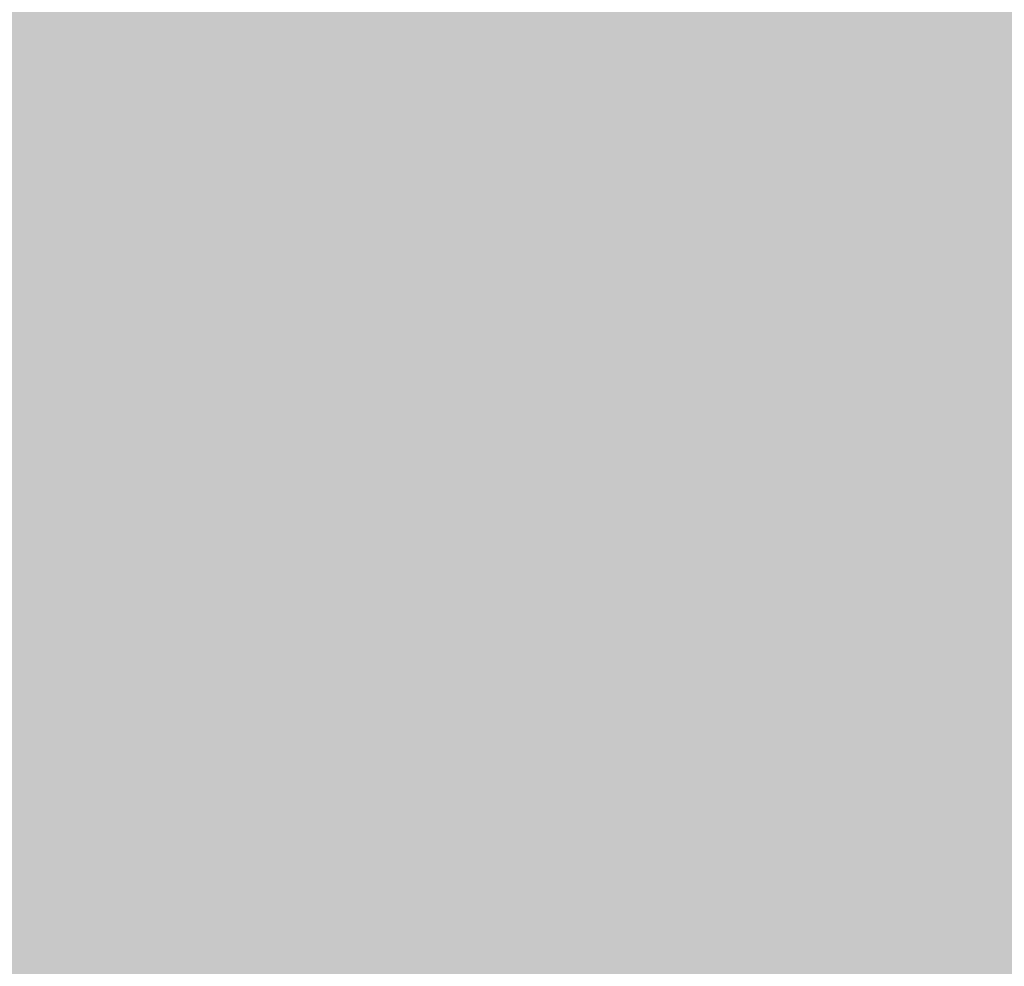
# Model space of a CAD drawing. Units: inches. Extents: x 2083 to 3317, y 1141 to 2115.
# Tile 140 of 256: x 3126.1318 to 3126.6699, y 1263.6134 to 1264.1307. Entities that reach past the tile are written whole.
import ezdxf

# ---------------------------------------------------------------- set-up
doc = ezdxf.new("R2010")
doc.units = ezdxf.units.IN
doc.layers.add('A-ANNO-DIMS', color=2, linetype='Continuous', lineweight=18)
doc.layers.add('A-WALL-PATT', color=251, linetype='Continuous', lineweight=13, true_color=0x636466)
doc.styles.get("Standard").update_dxf_attribs({"font": 'arial.ttf'})
doc.dimstyles.new('ISO-25', dxfattribs={"dimtxt": 12, "dimasz": 12, "dimexe": 1.25, "dimexo": 0.625, "dimtad": 1, "dimlunit": 3, "dimtxsty": 'Standard', "dimcen": 2.5, "dimadec": 0, "dimazin": 0, "dimtfac": 1, "dimtmove": 0, "dimatfit": 3, "dimfxl": 1, "dimarcsym": 0})

# ---------------------------------------------------------------- blocks, each defined once
blk = doc.blocks.new('*D26')
at = {"layer": 'A-ANNO-DIMS', "color": 0, "lineweight": -2, "transparency": 16777216}
for p, q in [((3088.98584, 1274.91509), (3088.98584, 1270.95196)), ((3111.24004, 1274.91509), (3111.24004, 1270.95196)), ((3076.98584, 1272.20196), (2840.26245, 1272.20196)), ((3111.24004, 1272.20196), (3088.98584, 1272.20196)), ((3123.24004, 1272.20196), (3135.24004, 1272.20196))]:
    blk.add_line(p, q, dxfattribs=at)
at = {"layer": 'A-ANNO-DIMS', "color": 0, "transparency": 16777216}
for points in [[(3076.98584, 1274.20196), (3076.98584, 1270.20196), (3088.98584, 1272.20196)], [(3123.24004, 1274.20196), (3123.24004, 1270.20196), (3111.24004, 1272.20196)]]:
    blk.add_solid(points, dxfattribs=at)
at = {"layer": 'Defpoints', "color": 0, "transparency": 16777216}
for p in [(3088.98584, 1275.54009), (3111.24004, 1275.54009), (3088.98584, 1272.20196)]:
    blk.add_point(p, dxfattribs=at)
at = {"layer": 'A-ANNO-DIMS', "color": 0, "transparency": 16777216, "insert": (2952.62415, 1279.0316), "char_height": 12, "attachment_point": 5}
blk.add_mtext('NIGHTSTAND 1\'-10 1/2" TYP.', dxfattribs=at)
blk = doc.blocks.new('*D27')
at = {"layer": 'A-ANNO-DIMS', "color": 0, "lineweight": -2, "transparency": 16777216}
for p, q in [((3114.57817, 1309.79428), (3114.57817, 1321.79428)), ((3111.86504, 1297.79428), (3115.82817, 1297.79428)), ((3114.57817, 1297.79428), (3114.57817, 1275.54009)), ((3111.86504, 1275.54009), (3115.82817, 1275.54009)), ((3114.57817, 1263.54009), (3114.57817, 1140.98859))]:
    blk.add_line(p, q, dxfattribs=at)
at = {"layer": 'A-ANNO-DIMS', "color": 0, "transparency": 16777216}
for points in [[(3112.57817, 1309.79428), (3116.57817, 1309.79428), (3114.57817, 1297.79428)], [(3112.57817, 1263.54009), (3116.57817, 1263.54009), (3114.57817, 1275.54009)]]:
    blk.add_solid(points, dxfattribs=at)
at = {"layer": 'Defpoints', "color": 0, "transparency": 16777216}
for p in [(3111.24004, 1297.79428), (3111.24004, 1275.54009), (3114.57817, 1275.54009)]:
    blk.add_point(p, dxfattribs=at)
at = {"layer": 'A-ANNO-DIMS', "color": 0, "transparency": 16777216, "insert": (3107.74853, 1196.26434), "char_height": 12, "attachment_point": 5, "rotation": 90}
blk.add_mtext('1\'-10 1/2" TYP.', dxfattribs=at)

msp = doc.modelspace()

# ---------------------------------------------------------------- hatches: boundary and pattern name
at = {"layer": 'A-WALL-PATT'}
h = msp.add_hatch(color=256, dxfattribs=at)
h.dxf.hatch_style = 1
h.paths.add_polyline_path([(3126.95978, 2020.76136), (2748.95978, 2020.76136), (2604.95978, 2020.76136), (2226.95978, 2020.76136), (2226.95978, 1702.76136), (2466.95978, 1702.76136), (2466.95978, 1582.76136), (2418.95978, 1582.76136), (2418.95978, 1477.76136), (2226.95978, 1477.76136), (2226.95978, 1263.26136), (2544.95978, 1263.26136), (2544.95978, 1411.76136), (2604.95978, 1411.76136), (2685.95978, 1411.76136), (2685.95978, 1420.76136), (2604.95978, 1420.76136), (2604.95978, 1573.76136), (2604.95978, 1702.76136), (2604.95978, 2011.76136), (2748.95978, 2011.76136), (2748.95978, 1702.76136), (2862.95978, 1702.76136), (2862.95978, 1621.76136), (2871.95978, 1621.76136), (2871.95978, 1702.76136), (2883.95978, 1702.76136), (2883.95978, 1706.93946, -0.026459), (2883.95978, 1711.76136), (2757.95978, 1711.76136), (2757.95978, 1807.76136), (2787.95978, 1807.76136), (2787.95978, 1812.26136), (2757.95978, 1812.26136), (2757.95978, 2011.76136), (2877.95978, 2011.76136), (2877.95978, 1812.26136), (2847.95978, 1812.26136), (2847.95978, 1807.76136), (2889.83574, 1807.76136), (2889.83574, 1812.26136), (2882.45978, 1812.26136), (2882.45978, 2011.76136), (3117.95978, 2011.76136), (3117.95978, 1812.26136), (2937.83574, 1812.26136), (2937.83574, 1807.76136), (2995.70978, 1807.76136), (2995.70978, 1796.11767), (3000.20978, 1796.11767), (3000.20978, 1807.76136), (3117.95978, 1807.76136), (3117.95978, 1711.76136), (3000.20978, 1711.76136), (3000.20978, 1760.11767), (2998.5727, 1760.11767, -0.020711), (2995.70978, 1760.11767), (2995.70978, 1711.76136), (2931.95978, 1711.76136), (2931.95978, 1702.76136), (3126.95978, 1702.76136)])
h.paths.add_polyline_path([(2471.45978, 2011.76136), (2471.45978, 1810.01136), (2462.71694, 1810.01136), (2462.71694, 1805.51136), (2505.95978, 1805.51136), (2505.95978, 1810.01136), (2475.95978, 1810.01136), (2475.95978, 2011.76136), (2595.95978, 2011.76136), (2595.95978, 1810.01136), (2565.95978, 1810.01136), (2565.95978, 1805.51136), (2595.95978, 1805.51136), (2595.95978, 1711.76136), (2235.95978, 1711.76136), (2235.95978, 1805.51136), (2353.70978, 1805.51136), (2353.70978, 1796.05416), (2358.20978, 1796.05416), (2358.20978, 1805.51136), (2414.71694, 1805.51136), (2414.71694, 1810.01136), (2235.95978, 1810.01136), (2235.95978, 2011.76136)], flags=16)
h.paths.add_polyline_path([(2270.20473, 1994.61001), (2270.20473, 1970.61001), (2246.20473, 1970.61001), (2246.20473, 1994.61001)], flags=0)
edge = h.paths.add_edge_path(flags=0)
edge.add_ellipse((2332.02739, 1899.79818), major_axis=(-3.04299, 3.04299), ratio=0.1682525, start_angle=-161.33217, end_angle=-156.30711, ccw=False)
edge.add_ellipse((2333.08204, 1898.74353), major_axis=(-1.05465, 1.05465), ratio=0.4535321, start_angle=-123.37102, end_angle=-94.15911)
edge = h.paths.add_edge_path(flags=0)
edge.add_ellipse((2332.02739, 1968.87629), major_axis=(3.04299, 3.04299), ratio=0.1682525, start_angle=18.66783, end_angle=23.69289)
edge.add_spline(control_points=[(2332.9256, 1970.6911), (2332.22677, 1970.3361), (2330.89371, 1969.65891), (2328.41308, 1970.93214), (2327.20393, 1967.74871), (2324.7096, 1969.95559), (2322.53282, 1967.01235), (2320.01285, 1971.29581), (2317.68031, 1968.15784), (2316.04053, 1967.10205), (2315.4269, 1966.8096)], knot_values=[0, 0, 0, 0, 2.267059, 4.324559, 6.685584, 8.878641, 11.121502, 14.300359, 17.755284, 19.732645, 19.732645, 19.732645, 19.732645], degree=3, periodic=0)
edge.add_ellipse((2332.02739, 1968.87629), major_axis=(3.04299, 3.04299), ratio=0.1682525, start_angle=18.66783, end_angle=23.69289, ccw=False)
edge.add_ellipse((2333.08204, 1969.93094), major_axis=(1.05465, 1.05465), ratio=0.4535321, start_angle=56.62898, end_angle=85.84089, ccw=False)
edge = h.paths.add_edge_path(flags=0)
edge.add_spline(control_points=[(2296.42829, 1967.98791), (2293.6278, 1965.33631), (2287.70362, 1959.72709), (2299.74386, 1949.9957), (2294.53259, 1935.66853), (2290.57323, 1920.60351), (2293.39412, 1909.97369), (2296.18541, 1904.96654)], knot_values=[0.099185, 0.099185, 0.099185, 0.099185, 0.345301, 0.619822, 0.982653, 1.386093, 1.810555, 1.810555, 1.810555, 1.810555], degree=3, periodic=0)
edge.add_spline(control_points=[(2296.18541, 1904.96654), (2297.38358, 1902.6193), (2298.00097, 1901.94931), (2298.55297, 1901.46815)], knot_values=[0.006246, 0.006246, 0.006246, 0.006246, 0.055476, 0.055476, 0.055476, 0.055476], degree=3, periodic=0)
edge.add_spline(control_points=[(2298.55297, 1901.46815), (2297.25861, 1900.92322), (2295.22529, 1900.23213), (2293.06023, 1900.61421), (2292.10142, 1900.78841), (2292.08958, 1900.79057)], knot_values=[0.312835, 0.312835, 0.312835, 0.312835, 0.40178, 0.474987, 0.475903, 0.475903, 0.475903, 0.475903], degree=3, periodic=0)
edge.add_arc((2292.79365, 1904.66411), 3.93701, 215.4209, 259.69818, ccw=False)
edge.add_spline(control_points=[(2289.58531, 1902.3823), (2289.47665, 1902.53509), (2289.36848, 1902.68804), (2289.26086, 1902.84117)], knot_values=[0.102872, 0.102872, 0.102872, 0.102872, 0.116896, 0.116896, 0.116896, 0.116896], degree=3, periodic=0)
edge.add_spline(control_points=[(2289.26086, 1902.84117), (2288.6866, 1902.55019), (2287.64005, 1902.0199), (2285.88134, 1901.87395), (2283.85297, 1901.50435), (2281.71999, 1899.71054), (2278.46699, 1899.49294), (2276.15714, 1901.8832), (2272.25895, 1899.80407), (2267.77761, 1901.84318), (2262.24388, 1900.18403), (2257.41493, 1901.78206), (2254.31837, 1900.72612), (2253.17828, 1900.33734)], knot_values=[0, 0, 0, 0, 1.907977, 3.477176, 5.261074, 7.972851, 11.680248, 13.717921, 16.939592, 22.789562, 27.502503, 33.595215, 37.145618, 37.145618, 37.145618, 37.145618], degree=3, periodic=0)
edge.add_line((2253.17828, 1900.33734), (2250.24424, 1902.84117))
edge.add_line((2250.24424, 1902.84117), (2250.24424, 1965.8333))
edge.add_line((2250.24424, 1965.8333), (2253.17828, 1968.33712))
edge.add_spline(control_points=[(2253.17828, 1968.33712), (2254.31837, 1967.94835), (2257.41493, 1966.89241), (2262.24388, 1968.49043), (2267.77761, 1966.83128), (2271.52673, 1968.53722), (2273.87591, 1967.82829), (2274.2067, 1967.72764)], knot_values=[0, 0, 0, 0, 0.09018, 0.244935, 0.364644, 0.513233, 0.537855, 0.537855, 0.537855, 0.537855], degree=3, periodic=0)
edge.add_arc((2274.35289, 1963.79335), 3.93701, 72.05113, 92.12795, ccw=False)
edge.add_arc((2281.29693, 1985.23), 18.5963, 252.051134, 288.565722)
edge.add_arc((2292.31672, 1956.02888), 12.64608, 71.026788, 113.778218, ccw=False)
edge = h.paths.add_edge_path(flags=0)
edge.add_spline(control_points=[(2274.89941, 1951.85619), (2275.06616, 1951.61659), (2275.23269, 1951.37659), (2275.39799, 1951.13585)], knot_values=[1.409916, 1.409916, 1.409916, 1.409916, 1.43159, 1.43159, 1.43159, 1.43159], degree=3, periodic=0)
edge.add_spline(control_points=[(2275.39799, 1951.13585), (2275.79211, 1950.56189), (2276.17923, 1949.98377), (2276.54555, 1949.3971)], knot_values=[1.358238, 1.358238, 1.358238, 1.358238, 1.409916, 1.409916, 1.409916, 1.409916], degree=3, periodic=0)
edge.add_line((2276.54555, 1949.3971), (2277.43729, 1947.86218))
edge.add_spline(control_points=[(2277.43729, 1947.86218), (2276.30383, 1945.67311), (2274.6397, 1942.42688), (2274.63161, 1938.0939), (2272.79912, 1930.85155), (2274.35643, 1943.89705), (2275.94768, 1947.92336), (2276.54555, 1949.3971)], knot_values=[0.005632, 0.005632, 0.005632, 0.005632, 0.186014, 0.266002, 0.357087, 0.59639, 0.739732, 0.739732, 0.739732, 0.739732], degree=3, periodic=0)
edge.add_spline(control_points=[(2276.54555, 1949.3971), (2276.17923, 1949.98377), (2275.79211, 1950.56189), (2275.39799, 1951.13585)], knot_values=[1.358238, 1.358238, 1.358238, 1.358238, 1.409916, 1.409916, 1.409916, 1.409916], degree=3, periodic=0)
edge.add_spline(control_points=[(2275.39799, 1951.13585), (2274.9425, 1950.08045), (2274.20776, 1948.02527), (2273.9346, 1944.85148), (2272.46853, 1937.62749), (2273.46622, 1945.69647), (2274.70062, 1951.05947), (2274.89941, 1951.85619)], knot_values=[0.104364, 0.104364, 0.104364, 0.104364, 0.189636, 0.269624, 0.36071, 0.600013, 0.644622, 0.644622, 0.644622, 0.644622], degree=3, periodic=0)
h.paths.add_polyline_path([(2269.16751, 1963.12757, -0.357527), (2268.17063, 1960.97637, -0.092561), (2268.17063, 1939.43632, -0.357527), (2269.16751, 1937.28512, -0.357527), (2267.01631, 1938.282, -0.164785), (2254.68558, 1938.282, -0.357527), (2252.53438, 1937.28512, -0.357527), (2253.53126, 1939.43632, -0.092561), (2253.53126, 1960.97637, -0.357527), (2252.53438, 1963.12757, -0.357527), (2254.68558, 1962.13069, -0.164785), (2267.01631, 1962.13069, -0.357527)], flags=0)
h.paths.add_polyline_path([(2248.87407, 1967.8018), (2248.87407, 1957.02771), (2249.45778, 1957.02771), (2249.45778, 1911.64676), (2248.87407, 1911.64676), (2248.87407, 1900.87267), (2246.51186, 1900.87267, 0.197327), (2244.14966, 1902.45687), (2244.14966, 1966.21759, 0.197327), (2246.51186, 1967.8018)], flags=0)
h.paths.add_polyline_path([(2269.16751, 1931.38934, -0.357527), (2268.17063, 1929.23814, -0.092561), (2268.17063, 1907.6981, -0.357527), (2269.16751, 1905.54689, -0.357527), (2267.01631, 1906.54377, -0.164785), (2254.68558, 1906.54377, -0.357527), (2252.53438, 1905.54689, -0.357527), (2253.53126, 1907.6981, -0.092561), (2253.53126, 1929.23814, -0.357527), (2252.53438, 1931.38934, -0.357527), (2254.68558, 1930.39246, -0.164785), (2267.01631, 1930.39246, -0.357527)], flags=0)
edge = h.paths.add_edge_path(flags=0)
edge.add_spline(control_points=[(2276.19686, 1906.7237), (2276.16814, 1909.02893), (2276.11405, 1913.37185), (2270.59842, 1924.92498), (2273.90517, 1919.01278), (2275.92171, 1916.26206), (2275.47457, 1912.40215), (2277.25787, 1910.38062), (2276.69604, 1908.22504), (2276.64622, 1906.81302), (2276.61782, 1906.00841)], knot_values=[0, 0, 0, 0, 8.61026, 16.221274, 18.843057, 23.804898, 27.440828, 29.356102, 31.203478, 33.650687, 33.650687, 33.650687, 33.650687], degree=3, periodic=0)
edge.add_spline(control_points=[(2276.61782, 1906.00841), (2276.62331, 1905.62414), (2276.49774, 1904.62866), (2275.44178, 1903.85473), (2274.93731, 1903.08045), (2274.85908, 1902.84117)], knot_values=[0.156488, 0.156488, 0.156488, 0.156488, 0.184398, 0.231376, 0.250598, 0.250598, 0.250598, 0.250598], degree=3, periodic=0)
edge.add_line((2274.85908, 1902.84117), (2276.50598, 1902.84117))
edge.add_spline(control_points=[(2276.50598, 1902.84117), (2276.78831, 1903.08494), (2277.66507, 1904.1252), (2278.24954, 1904.34074), (2277.65387, 1908.52739), (2278.15567, 1906.22781), (2278.10046, 1905.28595), (2278.84667, 1904.06901), (2277.85679, 1903.41495), (2277.87419, 1902.99105), (2277.90356, 1902.84117)], knot_values=[0.059574, 0.059574, 0.059574, 0.059574, 0.080753, 0.103741, 0.16972, 0.176036, 0.207137, 0.240474, 0.262341, 0.27366, 0.27366, 0.27366, 0.27366], degree=3, periodic=0)
edge.add_line((2277.90356, 1902.84117), (2280.02983, 1902.84117))
edge.add_spline(control_points=[(2280.02983, 1902.84117), (2279.88822, 1903.0884), (2279.49926, 1903.98155), (2280.15228, 1905.93935), (2278.10362, 1909.65776), (2279.76239, 1907.18529), (2280.3279, 1904.87486), (2280.48511, 1903.48959), (2281.46327, 1903.24943), (2281.75834, 1902.9365), (2281.83404, 1902.84117)], knot_values=[0.013856, 0.013856, 0.013856, 0.013856, 0.034874, 0.088867, 0.107879, 0.126738, 0.158714, 0.193757, 0.217487, 0.226722, 0.226722, 0.226722, 0.226722], degree=3, periodic=0)
edge.add_spline(control_points=[(2281.83404, 1902.84117), (2281.78753, 1902.8267), (2281.64702, 1902.78299), (2281.39553, 1902.85949), (2281.08808, 1902.98524), (2280.72068, 1903.0609), (2280.33345, 1903.02573), (2280.12477, 1902.89888), (2280.02983, 1902.84117)], knot_values=[0, 0, 0, 0, 0.14413, 0.435517, 0.749276, 1.153046, 1.548371, 1.878348, 1.878348, 1.878348, 1.878348], degree=3, periodic=0)
edge.add_line((2280.02983, 1902.84117), (2277.90356, 1902.84117))
edge.add_spline(control_points=[(2277.90356, 1902.84117), (2277.89286, 1902.79586), (2277.8654, 1902.67964), (2277.60748, 1902.68748), (2277.27405, 1902.8007), (2276.83792, 1902.61977), (2276.58381, 1902.78926), (2276.50598, 1902.84117)], knot_values=[0, 0, 0, 0, 0.127189, 0.326199, 0.628009, 1.24357, 1.515331, 1.515331, 1.515331, 1.515331], degree=3, periodic=0)
edge.add_line((2276.50598, 1902.84117), (2274.85908, 1902.84117))
edge.add_spline(control_points=[(2274.85908, 1902.84117), (2274.81444, 1902.89859), (2274.72513, 1903.01345), (2274.49348, 1903.11897), (2274.24429, 1902.96054), (2273.93712, 1903.18494), (2273.61404, 1902.98314), (2273.40832, 1902.88304), (2273.32225, 1902.84117)], knot_values=[0, 0, 0, 0, 0.21843, 0.436957, 0.687977, 0.990379, 1.398396, 1.69185, 1.69185, 1.69185, 1.69185], degree=3, periodic=0)
edge.add_spline(control_points=[(2273.32225, 1902.84117), (2273.61674, 1903.44569), (2274.274, 1904.53825), (2276.02724, 1904.5737), (2276.20696, 1906.58364), (2276.19686, 1906.7237)], knot_values=[0.012227, 0.012227, 0.012227, 0.012227, 0.059472, 0.106218, 0.134458, 0.134458, 0.134458, 0.134458], degree=3, periodic=0)
h.paths.add_polyline_path([(2270.77605, 1897.78983), (2270.77605, 1873.78983), (2246.77605, 1873.78983), (2246.77605, 1897.78983)], flags=0)
h.paths.add_polyline_path([(2353.70978, 1760.00506), (2353.70978, 1760.05416), (2358.20978, 1760.05416, -0.033729)], flags=0)
h.paths.add_polyline_path([(2321.81912, 1737.52919), (2341.99533, 1737.52919, -0.414214), (2343.20327, 1736.32124), (2343.20327, 1721.0206, -0.414214), (2341.99533, 1719.81265), (2321.81912, 1719.81265, -0.414214), (2320.61117, 1721.0206), (2320.61117, 1736.32124, -0.414214)], flags=0)
h.paths.add_polyline_path([(2324.23501, 1736.32124), (2339.57944, 1736.32124, -0.414214), (2341.99533, 1733.90535), (2341.99533, 1725.44973, -0.414214), (2339.57944, 1723.03384), (2333.68059, 1723.03384), (2333.84532, 1722.04547, -0.870646), (2335.4254, 1721.82589, -0.767327), (2333.92269, 1721.42324), (2331.29102, 1721.42324, -0.767327), (2329.78832, 1721.82589, -0.870646), (2331.3684, 1722.04547), (2331.53313, 1723.03384), (2324.23501, 1723.03384, -0.414214), (2321.81912, 1725.44973), (2321.81912, 1733.90535, -0.414214)], flags=0)
h.paths.add_polyline_path([(2570.48379, 1928.61544), (2589.68379, 1928.61544), (2590.16883, 1928.61544), (2590.16883, 1904.9934), (2570.48379, 1904.9934)], flags=0)
h.paths.add_polyline_path([(2574.44732, 1927.26382, -1), (2572.82884, 1927.26382, -1)], flags=0)
h.paths.add_polyline_path([(2573.08987, 1926.94088), (2573.92503, 1927.77604), (2574.14774, 1927.55333), (2573.31258, 1926.71817)], flags=0)
h.paths.add_polyline_path([(2578.77906, 1919.72962, -1), (2571.59166, 1919.72962, -1)], flags=0)
h.paths.add_polyline_path([(2578.38536, 1919.72962, -1), (2571.98536, 1919.72962, -1)], flags=0)
h.paths.add_polyline_path([(2331.59576, 1729.47622, -1), (2333.61795, 1729.47622, -1)], flags=0)
h.paths.add_polyline_path([(2578.03423, 1927.26382, -1), (2576.41574, 1927.26382, -1)], flags=0)
h.paths.add_polyline_path([(2576.68885, 1927.53109), (2576.91156, 1927.7538), (2577.74673, 1926.91863), (2577.52402, 1926.69592)], flags=0)
h.paths.add_polyline_path([(2578.13906, 1909.85954, -1), (2572.23166, 1909.85954, -1)], flags=0)
h.paths.add_polyline_path([(2577.74536, 1909.85954, -1), (2572.62536, 1909.85954, -1)], flags=0)
h.paths.add_polyline_path([(2583.79772, 1927.26382, -1), (2582.17923, 1927.26382, -1)], flags=0)
h.paths.add_polyline_path([(2582.71865, 1927.7538), (2583.55381, 1926.91863), (2583.3311, 1926.69592), (2582.49594, 1927.53109)], flags=0)
h.paths.add_polyline_path([(2582.49594, 1927.53109), (2582.71865, 1927.7538), (2583.55381, 1926.91863), (2583.3311, 1926.69592)], flags=0)
h.paths.add_polyline_path([(2587.73906, 1920.52962, -1), (2581.83166, 1920.52962, -1)], flags=0)
h.paths.add_polyline_path([(2587.34536, 1920.52962, -1), (2582.22536, 1920.52962, -1)], flags=0)
h.paths.add_polyline_path([(2587.38462, 1927.26382, -1), (2585.76613, 1927.26382, -1)], flags=0)
h.paths.add_polyline_path([(2586.08199, 1926.98025), (2586.91716, 1927.81541), (2587.13987, 1927.5927), (2586.3047, 1926.75754)], flags=0)
h.paths.add_polyline_path([(2588.37906, 1910.65954, -1), (2581.19166, 1910.65954, -1)], flags=0)
h.paths.add_polyline_path([(2587.98536, 1910.65954, -1), (2581.58536, 1910.65954, -1)], flags=0)
h.paths.add_polyline_path([(2417.16773, 1729.4779), (2437.34394, 1729.4779, -0.414214), (2438.55188, 1728.26995), (2438.55188, 1712.96931, -0.414214), (2437.34394, 1711.76136), (2417.16773, 1711.76136, -0.414214), (2415.95978, 1712.96931), (2415.95978, 1728.26995, -0.414214)], flags=0)
h.paths.add_polyline_path([(2419.58362, 1728.26995), (2434.92805, 1728.26995, -0.414214), (2437.34394, 1725.85406), (2437.34394, 1717.39844, -0.414214), (2434.92805, 1714.98255), (2429.0292, 1714.98255), (2429.19393, 1713.99418, -0.870646), (2430.77401, 1713.7746, -0.767327), (2429.2713, 1713.37195), (2426.63963, 1713.37195, -0.767327), (2425.13693, 1713.7746, -0.870646), (2426.71701, 1713.99418), (2426.88174, 1714.98255), (2419.58362, 1714.98255, -0.414214), (2417.16773, 1717.39844), (2417.16773, 1725.85406, -0.414214)], flags=0)
h.paths.add_polyline_path([(2419.58362, 1728.26995), (2434.92805, 1728.26995, -0.414214), (2437.34394, 1725.85406), (2437.34394, 1717.39844, -0.414214), (2434.92805, 1714.98255), (2429.0292, 1714.98255), (2428.35812, 1719.00903), (2427.55282, 1719.00903), (2426.88174, 1714.98255), (2419.58362, 1714.98255, -0.414214), (2417.16773, 1717.39844), (2417.16773, 1725.85406, -0.414214)], flags=0)
h.paths.add_polyline_path([(2426.94437, 1721.42492, -1), (2428.96656, 1721.42492, -1)], flags=0)
h.paths.add_polyline_path([(2475.95978, 1702.76136), (2595.95978, 1702.76136), (2595.95978, 1582.76136), (2475.95978, 1582.76136)], flags=16)
h.paths.add_polyline_path([(2427.95978, 1573.76136), (2595.95978, 1573.76136), (2595.95978, 1468.76136), (2595.95978, 1420.76136), (2384.45978, 1420.76136), (2384.45978, 1468.76136), (2427.95978, 1468.76136)], flags=16)
h.paths.add_polyline_path([(2379.95978, 1468.76136), (2379.95978, 1420.76136), (2235.95978, 1420.76136), (2235.95978, 1468.76136)], flags=16)
h.paths.add_polyline_path([(2317.816, 1466.69577), (2337.9922, 1466.69577, -0.414214), (2339.20015, 1465.48782), (2339.20015, 1450.18718, -0.414214), (2337.9922, 1448.97923), (2317.816, 1448.97923, -0.414214), (2316.60805, 1450.18718), (2316.60805, 1465.48782, -0.414214)], flags=0)
h.paths.add_polyline_path([(2320.23189, 1465.48782), (2335.57631, 1465.48782, -0.414214), (2337.9922, 1463.07193), (2337.9922, 1454.61631, -0.414214), (2335.57631, 1452.20042), (2329.67747, 1452.20042), (2329.84219, 1451.21205, -0.870646), (2331.42228, 1450.99247, -0.767327), (2329.91957, 1450.58983), (2327.2879, 1450.58983, -0.767327), (2325.7852, 1450.99247, -0.870646), (2327.36528, 1451.21205), (2327.53001, 1452.20042), (2320.23189, 1452.20042, -0.414214), (2317.816, 1454.61631), (2317.816, 1463.07193, -0.414214)], flags=0)
h.paths.add_polyline_path([(2320.23189, 1465.48782), (2335.57631, 1465.48782, -0.414214), (2337.9922, 1463.07193), (2337.9922, 1454.61631, -0.414214), (2335.57631, 1452.20042), (2329.67747, 1452.20042), (2329.00638, 1456.22691), (2328.20109, 1456.22691), (2327.53001, 1452.20042), (2320.23189, 1452.20042, -0.414214), (2317.816, 1454.61631), (2317.816, 1463.07193, -0.414214)], flags=0)
h.paths.add_polyline_path([(2327.59264, 1458.6428, -1), (2329.61483, 1458.6428, -1)], flags=0)
h.paths.add_polyline_path([(2244.41174, 1433.34045), (2241.92094, 1433.34045, -0.414214), (2240.01786, 1435.24354), (2240.01786, 1440.95281, -0.414211), (2241.92093, 1442.8559), (2244.41174, 1442.8559, -1.976472)], flags=0)
h.paths.add_polyline_path([(2245.35689, 1434.39754, -0.414214), (2245.35689, 1441.79881, -2.144098)], flags=0)
h.paths.add_polyline_path([(2535.95978, 1416.26136), (2535.95978, 1272.26136), (2235.95978, 1272.26136), (2235.95978, 1416.26136)], flags=16)
h.paths.add_polyline_path([(2260.11956, 1384.29284), (2260.11956, 1362.03865), (2237.86537, 1362.03865), (2237.86537, 1384.29284)], flags=0)
edge = h.paths.add_edge_path(flags=0)
edge.add_line((2318.25185, 1362.0933), (2318.1458, 1362.00097))
edge.add_ellipse((2317.44512, 1360.43104), major_axis=(2.82164, 2.82164), ratio=0.1682525, start_angle=18.66783, end_angle=20.94813, ccw=False)
edge.add_ellipse((2318.42305, 1361.40897), major_axis=(0.97793, 0.97793), ratio=0.4535321, start_angle=56.62898, end_angle=70.2262, ccw=False)
edge = h.paths.add_edge_path(flags=0)
edge.add_line((2319.10737, 1295.57108), (2319.01504, 1295.67713))
edge.add_ellipse((2317.44512, 1296.37781), major_axis=(-2.82164, 2.82164), ratio=0.1682525, start_angle=-161.33217, end_angle=-159.05187, ccw=False)
edge.add_ellipse((2318.42305, 1295.39988), major_axis=(-0.97793, 0.97793), ratio=0.4535321, start_angle=-123.37102, end_angle=-109.7738)
edge = h.paths.add_edge_path(flags=0)
edge.add_spline(control_points=[(2284.21035, 1301.17022), (2284.58069, 1300.44472), (2284.89119, 1299.89202), (2285.15955, 1299.46102)], knot_values=[0.039066, 0.039066, 0.039066, 0.039066, 0.055476, 0.055476, 0.055476, 0.055476], degree=3, periodic=0)
edge.add_line((2285.15955, 1299.46102), (2284.21035, 1301.17022))
edge = h.paths.add_edge_path(flags=0)
edge.add_line((2280.41246, 1297.29801), (2283.36999, 1297.03612))
edge.add_line((2283.36999, 1297.03612), (2286.40569, 1297.92631))
edge.add_spline(control_points=[(2286.40569, 1297.92631), (2285.30549, 1297.46312), (2284.34478, 1297.12915), (2283.36999, 1297.03612)], knot_values=[0.394369, 0.394369, 0.394369, 0.394369, 0.475903, 0.475903, 0.475903, 0.475903], degree=3, periodic=0)
edge.add_spline(control_points=[(2283.36999, 1297.03612), (2283.28139, 1297.02767), (2282.31629, 1296.95734), (2281.3125, 1297.13448), (2280.42344, 1297.29602), (2280.41246, 1297.29801)], knot_values=[0.312835, 0.312835, 0.312835, 0.312835, 0.320246, 0.393453, 0.394369, 0.394369, 0.394369, 0.394369], degree=3, periodic=0)
edge = h.paths.add_edge_path(flags=0)
edge.add_line((2284.43556, 1359.60729), (2280.44629, 1355.32805))
edge.add_line((2280.44629, 1355.32805), (2279.57999, 1351.01775))
edge.add_line((2279.57999, 1351.01775), (2282.41297, 1346.58043))
edge.add_spline(control_points=[(2282.41297, 1346.58043), (2283.15333, 1345.58924), (2284.2529, 1344.0289), (2284.80104, 1342.38717), (2284.93516, 1341.80554)], knot_values=[1.240098, 1.240098, 1.240098, 1.240098, 1.332892, 1.382712, 1.382712, 1.382712, 1.382712], degree=3, periodic=0)
edge.add_spline(control_points=[(2284.93516, 1341.80554), (2285.31911, 1340.1406), (2285.23303, 1338.4092), (2284.90994, 1336.65412)], knot_values=[1.097484, 1.097484, 1.097484, 1.097484, 1.240098, 1.240098, 1.240098, 1.240098], degree=3, periodic=0)
edge.add_spline(control_points=[(2284.90994, 1336.65412), (2284.58685, 1334.89904), (2284.02675, 1333.12027), (2283.46264, 1331.36058)], knot_values=[0.95487, 0.95487, 0.95487, 0.95487, 1.097484, 1.097484, 1.097484, 1.097484], degree=3, periodic=0)
edge.add_line((2283.46264, 1331.36058), (2281.89038, 1326.15336))
edge.add_line((2281.89038, 1326.15336), (2280.75626, 1321.05609))
edge.add_line((2280.75626, 1321.05609), (2280.2992, 1316.00198))
edge.add_line((2280.2992, 1316.00198), (2280.71593, 1310.95007))
edge.add_line((2280.71593, 1310.95007), (2282.02809, 1305.97214))
edge.add_line((2282.02809, 1305.97214), (2284.21035, 1301.17022))
edge.add_spline(control_points=[(2284.21035, 1301.17022), (2283.34073, 1302.73019), (2282.6119, 1304.33649), (2282.02809, 1305.97214)], knot_values=[0.099185, 0.099185, 0.099185, 0.099185, 0.241799, 0.241799, 0.241799, 0.241799], degree=3, periodic=0)
edge.add_spline(control_points=[(2282.02809, 1305.97214), (2281.44428, 1307.60778), (2281.00549, 1309.27276), (2280.71593, 1310.95007)], knot_values=[0.241799, 0.241799, 0.241799, 0.241799, 0.384413, 0.384413, 0.384413, 0.384413], degree=3, periodic=0)
edge.add_spline(control_points=[(2280.71593, 1310.95007), (2280.43324, 1312.58761), (2280.28939, 1314.27696), (2280.29889, 1315.96203), (2280.2992, 1316.00198)], knot_values=[0.384413, 0.384413, 0.384413, 0.384413, 0.523647, 0.527028, 0.527028, 0.527028, 0.527028], degree=3, periodic=0)
edge.add_spline(control_points=[(2280.2992, 1316.00198), (2280.31233, 1317.68696), (2280.47787, 1319.36793), (2280.75626, 1321.05609)], knot_values=[0.527028, 0.527028, 0.527028, 0.527028, 0.669642, 0.669642, 0.669642, 0.669642], degree=3, periodic=0)
edge.add_spline(control_points=[(2280.75626, 1321.05609), (2281.03465, 1322.74425), (2281.42588, 1324.43961), (2281.89038, 1326.15336)], knot_values=[0.669642, 0.669642, 0.669642, 0.669642, 0.812256, 0.812256, 0.812256, 0.812256], degree=3, periodic=0)
edge.add_spline(control_points=[(2281.89038, 1326.15336), (2282.26438, 1327.53325), (2282.78787, 1329.26181), (2283.35275, 1331.01778), (2283.46264, 1331.36058)], knot_values=[0.812256, 0.812256, 0.812256, 0.812256, 0.927087, 0.95487, 0.95487, 0.95487, 0.95487], degree=3, periodic=0)
edge.add_line((2283.46264, 1331.36058), (2284.90994, 1336.65412))
edge.add_line((2284.90994, 1336.65412), (2284.93516, 1341.80554))
edge.add_line((2284.93516, 1341.80554), (2282.41297, 1346.58043))
edge.add_spline(control_points=[(2282.41297, 1346.58043), (2281.27513, 1348.10379), (2280.07845, 1349.57032), (2279.57999, 1351.01775)], knot_values=[1.382712, 1.382712, 1.382712, 1.382712, 1.525326, 1.525326, 1.525326, 1.525326], degree=3, periodic=0)
edge.add_spline(control_points=[(2279.57999, 1351.01775), (2279.44328, 1351.41472), (2279.13631, 1352.85692), (2279.73519, 1354.29039), (2280.44629, 1355.32805)], knot_values=[1.525326, 1.525326, 1.525326, 1.525326, 1.564439, 1.667941, 1.667941, 1.667941, 1.667941], degree=3, periodic=0)
edge.add_spline(control_points=[(2280.44629, 1355.32805), (2281.42611, 1356.75784), (2282.93084, 1358.18256), (2284.43556, 1359.60729)], knot_values=[1.667941, 1.667941, 1.667941, 1.667941, 1.810555, 1.810555, 1.810555, 1.810555], degree=3, periodic=0)
edge.add_arc((2280.62307, 1348.51818), 11.72618, 71.026788, 113.778218)
edge.add_arc((2270.40489, 1375.59516), 17.24357, 252.051134, 288.565722, ccw=False)
edge.add_arc((2263.96597, 1355.71785), 3.65062, 72.05113, 92.12795)
edge.add_arc((2263.96597, 1355.71785), 3.65062, 92.12795, 177.98513)
edge.add_spline(control_points=[(2260.3176, 1355.8462), (2260.26042, 1354.22067), (2260.55128, 1350.18655), (2262.99934, 1346.76625), (2264.47274, 1344.64902)], knot_values=[1.43159, 1.43159, 1.43159, 1.43159, 1.564144, 1.770695, 1.770695, 1.770695, 1.770695], degree=3, periodic=0)
edge.add_line((2264.47274, 1344.64902), (2264.93559, 1343.98253))
edge.add_spline(control_points=[(2263.80104, 1340.24811), (2263.84324, 1340.51409), (2264.06724, 1341.75647), (2264.51269, 1343.00245), (2264.93505, 1343.98108)], knot_values=[0.53657, 0.53657, 0.53657, 0.53657, 0.559349, 0.644622, 0.644622, 0.644622, 0.644622], degree=3, periodic=0)
edge.add_spline(control_points=[(2264.93505, 1343.98108), (2265.11777, 1343.71497), (2265.29888, 1343.44791), (2265.47676, 1343.17936)], knot_values=[1.384077, 1.384077, 1.384077, 1.384077, 1.409916, 1.409916, 1.409916, 1.409916], degree=3, periodic=0)
edge.add_spline(control_points=[(2265.47676, 1343.17936), (2265.65464, 1342.91082), (2265.8293, 1342.64081), (2265.99913, 1342.36881)], knot_values=[1.358238, 1.358238, 1.358238, 1.358238, 1.384077, 1.384077, 1.384077, 1.384077], degree=3, periodic=0)
edge.add_line((2265.99913, 1342.36881), (2266.82601, 1340.94555))
edge.add_spline(control_points=[(2266.82601, 1340.94555), (2268.8944, 1337.08969), (2271.39817, 1325.843), (2270.51616, 1310.56856), (2275.91938, 1301.86061), (2277.78951, 1299.19945)], knot_values=[0.116896, 0.116896, 0.116896, 0.116896, 0.472987, 1.050969, 1.313793, 1.313793, 1.313793, 1.313793], degree=3, periodic=0)
edge.add_spline(control_points=[(2277.78951, 1299.19945), (2277.83941, 1299.12845), (2277.88943, 1299.0575), (2277.93957, 1298.98658)], knot_values=[0.109884, 0.109884, 0.109884, 0.109884, 0.116896, 0.116896, 0.116896, 0.116896], degree=3, periodic=0)
edge.add_line((2277.93957, 1298.98658), (2277.78885, 1299.19911))
edge.add_spline(control_points=[(2277.78885, 1299.19911), (2277.25658, 1298.92941), (2276.28635, 1298.4379), (2275.03935, 1298.33442), (2274.38333, 1298.2389), (2274.21525, 1298.20934)], knot_values=[33.12187, 33.12187, 33.12187, 33.12187, 35.029056, 36.598255, 37.144827, 37.144827, 37.144827, 37.144827], degree=3, periodic=0)
edge.add_line((2274.21525, 1298.20934), (2273.07315, 1297.89296))
edge.add_spline(control_points=[(2273.07315, 1297.89296), (2272.32294, 1297.57978), (2271.03915, 1296.51051), (2269.24839, 1296.22606), (2268.4231, 1296.37465)], knot_values=[26.532584, 26.532584, 26.532584, 26.532584, 29.198919, 31.839101, 31.839101, 31.839101, 31.839101], degree=3, periodic=0)
edge.add_line((2268.4231, 1296.37465), (2263.8785, 1297.45753))
edge.add_spline(control_points=[(2263.8785, 1297.45753), (2263.55608, 1297.35943), (2261.86031, 1296.83869), (2260.23878, 1297.28241), (2258.93345, 1297.51646)], knot_values=[15.919551, 15.919551, 15.919551, 15.919551, 16.939592, 21.226067, 21.226067, 21.226067, 21.226067], degree=3, periodic=0)
edge.add_line((2258.93345, 1297.51646), (2254.05523, 1297.32901))
edge.add_spline(control_points=[(2254.05523, 1297.32901), (2253.75553, 1297.29582), (2252.11368, 1297.16517), (2250.46187, 1297.54422), (2249.12969, 1297.66788)], knot_values=[5.306517, 5.306517, 5.306517, 5.306517, 6.276435, 10.613034, 10.613034, 10.613034, 10.613034], degree=3, periodic=0)
edge.add_line((2249.12969, 1297.66788), (2244.33165, 1296.87776))
edge.add_line((2244.33165, 1296.87776), (2241.61103, 1299.19945))
edge.add_line((2241.61103, 1299.19945), (2241.61103, 1357.6094))
edge.add_line((2241.61103, 1357.6094), (2244.33165, 1359.9311))
edge.add_line((2244.33165, 1359.9311), (2252.72882, 1359.54269))
edge.add_spline(control_points=[(2252.72882, 1359.54269), (2252.87094, 1359.54644), (2253.30574, 1359.54817), (2253.73984, 1359.51427), (2254.03174, 1359.48243)], knot_values=[0.233291, 0.233291, 0.233291, 0.233291, 0.244935, 0.268927, 0.268927, 0.268927, 0.268927], degree=3, periodic=0)
edge.add_line((2254.03174, 1359.48243), (2259.58719, 1359.41639))
edge.add_spline(control_points=[(2259.58719, 1359.41639), (2260.67707, 1359.6285), (2262.0732, 1359.897), (2263.52369, 1359.45928), (2263.83042, 1359.36595)], knot_values=[0.422516, 0.422516, 0.422516, 0.422516, 0.513233, 0.537855, 0.537855, 0.537855, 0.537855], degree=3, periodic=0)
edge.add_arc((2263.96597, 1355.71785), 3.65062, 72.05113, 92.12795, ccw=False)
edge.add_arc((2270.40489, 1375.59516), 17.24357, 252.051134, 288.565722)
edge.add_arc((2280.62307, 1348.51818), 11.72618, 71.026788, 113.778218, ccw=False)
h.paths.add_polyline_path([(2240.34053, 1359.43471), (2240.34053, 1349.44435), (2240.88178, 1349.44435), (2240.88178, 1307.3645), (2240.34053, 1307.3645), (2240.34053, 1297.37414), (2238.15016, 1297.37414, 0.197327), (2235.95978, 1298.84311), (2235.95978, 1357.96575, 0.197327), (2238.15016, 1359.43471)], flags=0)
h.paths.add_polyline_path([(2259.15779, 1355.1005, -0.357527), (2258.23342, 1353.10578, -0.092561), (2258.23342, 1333.1326, -0.357527), (2259.15779, 1331.13788, -0.357527), (2257.16307, 1332.06225, -0.164785), (2245.7293, 1332.06225, -0.357527), (2243.73458, 1331.13788, -0.357527), (2244.65895, 1333.1326, -0.092561), (2244.65895, 1353.10578, -0.357527), (2243.73458, 1355.1005, -0.357527), (2245.7293, 1354.17613, -0.164785), (2257.16307, 1354.17613, -0.357527)], flags=0)
edge = h.paths.add_edge_path(flags=0)
edge.add_line((2265.99913, 1342.36881), (2266.82601, 1340.94555))
edge.add_line((2266.82601, 1340.94555), (2265.30756, 1337.81407))
edge.add_line((2265.30756, 1337.81407), (2264.35823, 1334.65294))
edge.add_line((2264.35823, 1334.65294), (2264.26201, 1333.7997))
edge.add_spline(control_points=[(2264.26201, 1333.7997), (2264.20836, 1333.18705), (2264.16206, 1332.36553), (2264.00714, 1331.41393), (2263.96905, 1331.20183)], knot_values=[0.464444, 0.464444, 0.464444, 0.464444, 0.516691, 0.531608, 0.531608, 0.531608, 0.531608], degree=3, periodic=0)
edge.add_spline(control_points=[(2263.96905, 1331.20183), (2263.77453, 1330.11887), (2263.42437, 1328.79084), (2263.25742, 1328.53065), (2263.23403, 1328.51461)], knot_values=[0.372682, 0.372682, 0.372682, 0.372682, 0.44885, 0.464444, 0.464444, 0.464444, 0.464444], degree=3, periodic=0)
edge.add_spline(control_points=[(2263.23403, 1328.51461), (2263.09638, 1328.42023), (2263.13117, 1329.30148), (2263.27495, 1330.61575)], knot_values=[0.280919, 0.280919, 0.280919, 0.280919, 0.372682, 0.372682, 0.372682, 0.372682], degree=3, periodic=0)
edge.add_spline(control_points=[(2263.27495, 1330.61575), (2263.41874, 1331.93002), (2263.67152, 1333.67732), (2263.96985, 1335.31503)], knot_values=[0.189157, 0.189157, 0.189157, 0.189157, 0.280919, 0.280919, 0.280919, 0.280919], degree=3, periodic=0)
edge.add_spline(control_points=[(2263.96985, 1335.31503), (2264.1005, 1336.03219), (2264.41878, 1337.62191), (2264.75485, 1338.86443), (2264.94742, 1339.49112)], knot_values=[0.097394, 0.097394, 0.097394, 0.097394, 0.137578, 0.189157, 0.189157, 0.189157, 0.189157], degree=3, periodic=0)
edge.add_spline(control_points=[(2264.94742, 1339.49112), (2265.29002, 1340.60605), (2265.64424, 1341.494), (2265.99913, 1342.36881)], knot_values=[0.005632, 0.005632, 0.005632, 0.005632, 0.097394, 0.097394, 0.097394, 0.097394], degree=3, periodic=0)
h.paths.add_polyline_path([(2259.15779, 1325.67097, -0.357527), (2258.23342, 1323.67625, -0.092561), (2258.23342, 1303.70307, -0.357527), (2259.15779, 1301.70835, -0.357527), (2257.16307, 1302.63272, -0.164785), (2245.7293, 1302.63272, -0.357527), (2243.73458, 1301.70835, -0.357527), (2244.65895, 1303.70307, -0.092561), (2244.65895, 1323.67625, -0.357527), (2243.73458, 1325.67097, -0.357527), (2245.7293, 1324.74661, -0.164785), (2257.16307, 1324.74661, -0.357527)], flags=0)
edge = h.paths.add_edge_path(flags=0)
edge.add_spline(control_points=[(2261.70894, 1317.31142), (2261.67948, 1317.41758), (2261.76186, 1317.38853), (2262.49074, 1316.08987), (2262.96218, 1315.3009)], knot_values=[14.955861, 14.955861, 14.955861, 14.955861, 16.221274, 18.694826, 18.694826, 18.694826, 18.694826], degree=3, periodic=0)
edge.add_spline(control_points=[(2262.96218, 1315.3009), (2262.99044, 1315.25362), (2263.7021, 1314.06738), (2264.34898, 1313.12715), (2264.73005, 1312.16415)], knot_values=[18.694826, 18.694826, 18.694826, 18.694826, 18.843057, 22.433791, 22.433791, 22.433791, 22.433791], degree=3, periodic=0)
edge.add_spline(control_points=[(2264.73005, 1312.16415), (2264.87556, 1311.79644), (2265.17687, 1310.76981), (2265.14307, 1309.55926), (2265.24774, 1308.82419)], knot_values=[22.433791, 22.433791, 22.433791, 22.433791, 23.804898, 26.172756, 26.172756, 26.172756, 26.172756], degree=3, periodic=0)
edge.add_line((2265.24774, 1308.82419), (2265.85077, 1307.17189))
edge.add_spline(control_points=[(2265.85077, 1307.17189), (2266.06502, 1306.82168), (2266.38439, 1306.33225), (2266.4244, 1305.78055), (2266.42037, 1305.61122)], knot_values=[28.062562, 28.062562, 28.062562, 28.062562, 29.356102, 29.911721, 29.911721, 29.911721, 29.911721], degree=3, periodic=0)
edge.add_spline(control_points=[(2266.42037, 1305.61122), (2266.41612, 1305.43259), (2266.394, 1305.25), (2266.36478, 1305.06586)], knot_values=[29.911721, 29.911721, 29.911721, 29.911721, 30.497837, 30.497837, 30.497837, 30.497837], degree=3, periodic=0)
edge.add_line((2266.36478, 1305.06586), (2266.06615, 1302.1363))
edge.add_spline(control_points=[(2266.06615, 1302.1363), (2266.07124, 1301.77998), (2265.99808, 1301.19998), (2265.66327, 1300.75896), (2265.50891, 1300.58588)], knot_values=[0.156488, 0.156488, 0.156488, 0.156488, 0.184398, 0.203543, 0.203543, 0.203543, 0.203543], degree=3, periodic=0)
edge.add_line((2265.50891, 1300.58588), (2264.43534, 1299.19945))
edge.add_line((2264.43534, 1299.19945), (2265.96244, 1299.19945))
edge.add_line((2265.96244, 1299.19945), (2267.33599, 1301.17528))
edge.add_line((2267.33599, 1301.17528), (2267.31167, 1301.98624))
edge.add_spline(control_points=[(2267.31167, 1301.98624), (2267.26111, 1302.8624), (2267.16021, 1303.73713), (2267.27149, 1303.3259)], knot_values=[0.126229, 0.126229, 0.126229, 0.126229, 0.166617, 0.166617, 0.166617, 0.166617], degree=3, periodic=0)
edge.add_spline(control_points=[(2267.27149, 1303.3259), (2267.28003, 1303.2943), (2267.30979, 1303.17537), (2267.37345, 1302.88361), (2267.40612, 1302.68283), (2267.41793, 1302.60103)], knot_values=[0.166617, 0.166617, 0.166617, 0.166617, 0.16972, 0.176036, 0.180765, 0.180765, 0.180765, 0.180765], degree=3, periodic=0)
edge.add_spline(control_points=[(2267.74389, 1300.9875), (2267.68758, 1301.15094), (2267.48052, 1301.65666), (2267.48375, 1302.14479), (2267.41793, 1302.60103)], knot_values=[0.180765, 0.180765, 0.180765, 0.180765, 0.193767, 0.220139, 0.220139, 0.220139, 0.220139], degree=3, periodic=0)
edge.add_line((2267.41793, 1302.60103), (2267.74389, 1300.9875))
edge.add_spline(control_points=[(2267.74389, 1300.9875), (2267.83196, 1300.73188), (2267.93202, 1300.3099), (2267.55484, 1299.97452), (2267.42937, 1299.82921)], knot_values=[0.220139, 0.220139, 0.220139, 0.220139, 0.240474, 0.25489, 0.25489, 0.25489, 0.25489], degree=3, periodic=0)
edge.add_line((2267.42937, 1299.82921), (2267.25836, 1299.19945))
edge.add_line((2267.25836, 1299.19945), (2269.22996, 1299.19945))
edge.add_spline(control_points=[(2269.22996, 1299.19945), (2269.09865, 1299.42869), (2268.84277, 1300.01625), (2269.01157, 1300.91592), (2268.9468, 1301.66074)], knot_values=[0.013856, 0.013856, 0.013856, 0.013856, 0.034874, 0.067073, 0.067073, 0.067073, 0.067073], degree=3, periodic=0)
edge.add_line((2268.9468, 1301.66074), (2268.43158, 1303.60311))
edge.add_spline(control_points=[(2268.43158, 1303.60311), (2268.1756, 1304.19237), (2267.59621, 1305.2513), (2268.0407, 1304.62321), (2268.25139, 1304.28242)], knot_values=[0.090155, 0.090155, 0.090155, 0.090155, 0.107879, 0.120289, 0.120289, 0.120289, 0.120289], degree=3, periodic=0)
edge.add_spline(control_points=[(2268.25139, 1304.28242), (2268.36088, 1304.10533), (2269.05775, 1302.91798), (2269.38269, 1301.59042), (2269.52141, 1300.77593), (2269.57522, 1300.55578)], knot_values=[0.120289, 0.120289, 0.120289, 0.120289, 0.126738, 0.158714, 0.173506, 0.173506, 0.173506, 0.173506], degree=3, periodic=0)
edge.add_line((2269.57522, 1300.55578), (2270.6858, 1299.42126))
edge.add_spline(control_points=[(2270.6858, 1299.42126), (2270.76722, 1299.35725), (2270.83785, 1299.2814), (2270.90292, 1299.19945)], knot_values=[0.21816, 0.21816, 0.21816, 0.21816, 0.226722, 0.226722, 0.226722, 0.226722], degree=3, periodic=0)
edge.add_line((2270.9372, 1299.19291), (2270.90292, 1299.19945))
edge.add_spline(control_points=[(2270.90292, 1299.19945), (2270.85981, 1299.18603), (2270.72951, 1299.1455), (2270.49631, 1299.21644), (2270.27166, 1299.30832), (2270.12102, 1299.34796), (2270.06334, 1299.35956)], knot_values=[0.939174, 0.939174, 0.939174, 0.939174, 1.083304, 1.374691, 1.68845, 1.878348, 1.878348, 1.878348, 1.878348], degree=3, periodic=0)
edge.add_line((2270.06334, 1299.35956), (2269.22996, 1299.19945))
edge.add_line((2269.22996, 1299.19945), (2267.25836, 1299.19945))
edge.add_spline(control_points=[(2267.25836, 1299.19945), (2267.24843, 1299.15743), (2267.22297, 1299.04967), (2266.98382, 1299.05694), (2266.80921, 1299.11623), (2266.6769, 1299.10909), (2266.63653, 1299.10481)], knot_values=[0.757665, 0.757665, 0.757665, 0.757665, 0.884854, 1.083864, 1.385675, 1.515331, 1.515331, 1.515331, 1.515331], degree=3, periodic=0)
edge.add_spline(control_points=[(2266.63653, 1299.10481), (2266.48522, 1299.08879), (2266.23581, 1299.01712), (2266.03461, 1299.15132), (2265.96244, 1299.19945)], knot_values=[0, 0, 0, 0, 0.485905, 0.757665, 0.757665, 0.757665, 0.757665], degree=3, periodic=0)
edge.add_line((2265.96244, 1299.19945), (2264.43534, 1299.19945))
edge.add_line((2264.43534, 1299.19945), (2263.85844, 1299.36712))
edge.add_spline(control_points=[(2263.85844, 1299.36712), (2263.81894, 1299.37091), (2263.77953, 1299.38572), (2263.74013, 1299.4015)], knot_values=[0.845925, 0.845925, 0.845925, 0.845925, 0.978627, 0.978627, 0.978627, 0.978627], degree=3, periodic=0)
edge.add_line((2263.72179, 1299.39643), (2263.01031, 1299.19945))
edge.add_spline(control_points=[(2263.01031, 1299.19945), (2263.24579, 1299.68286), (2263.50603, 1300.12811), (2263.87349, 1300.40803)], knot_values=[0.012227, 0.012227, 0.012227, 0.012227, 0.052971, 0.052971, 0.052971, 0.052971], degree=3, periodic=0)
edge.add_spline(control_points=[(2263.87349, 1300.40803), (2263.93213, 1300.4527), (2264.08424, 1300.55298), (2264.25519, 1300.62422), (2264.35969, 1300.66475)], knot_values=[0.052971, 0.052971, 0.052971, 0.052971, 0.059472, 0.069086, 0.069086, 0.069086, 0.069086], degree=3, periodic=0)
edge.add_line((2264.35969, 1300.66475), (2265.1419, 1301.07777))
edge.add_line((2265.1419, 1301.07777), (2265.67581, 1302.79956))
edge.add_line((2265.67581, 1302.79956), (2265.5407, 1305.70407))
edge.add_line((2265.5407, 1305.70407), (2264.80307, 1309.32772))
edge.add_line((2264.80307, 1309.32772), (2263.04053, 1314.09179))
edge.add_spline(control_points=[(2263.04053, 1314.09179), (2262.38357, 1315.67144), (2261.79597, 1316.99775), (2261.70894, 1317.31142)], knot_values=[11.216896, 11.216896, 11.216896, 11.216896, 14.955861, 14.955861, 14.955861, 14.955861], degree=3, periodic=0)
h.paths.add_polyline_path([(2871.95978, 1416.26136), (2895.91005, 1416.26136), (2895.91005, 1420.76136), (2871.95978, 1420.76136), (2871.95978, 1501.76136), (2862.95978, 1501.76136), (2862.95978, 1420.76136), (2805.95978, 1420.76136), (2805.95978, 1411.76136), (2862.95978, 1411.76136), (2862.95978, 1263.26136), (3126.95978, 1263.26136), (3126.95978, 1411.76136), (3126.95978, 1486.76136), (2943.95978, 1486.76136), (2943.95978, 1477.76136), (2967.86031, 1477.76136), (2967.86031, 1420.76136), (2943.91005, 1420.76136), (2943.91005, 1416.26136), (3117.95978, 1416.26136), (3117.95978, 1420.76136), (2972.36031, 1420.76136), (2972.36031, 1477.76136), (3117.95978, 1477.76136), (3117.95978, 1420.76136), (3117.95978, 1272.26136), (2871.95978, 1272.26136)], flags=0)
h.paths.add_polyline_path([(2457.12563, 1485.94251), (2527.60265, 1485.94251), (2527.60265, 1537.6357), (2457.12563, 1537.6357)], flags=8)
h.paths.add_polyline_path([(2481.00506, 1609.9818), (2590.76582, 1609.9818), (2590.76582, 1682.00336), (2481.00506, 1682.00336)], flags=8)
h.paths.add_polyline_path([(2483.08502, 1729.12678), (2553.56205, 1729.12678), (2553.56205, 1780.81998), (2483.08502, 1780.81998)], flags=8)
h = msp.add_hatch(color=256, dxfattribs=at)
h.dxf.hatch_style = 1
h.paths.add_polyline_path([(3126.95978, 1486.76136), (2943.95978, 1486.76136), (2943.95978, 1477.76136), (2967.86031, 1477.76136), (2967.86031, 1420.76136), (2943.91005, 1420.76136), (2943.91005, 1416.26136), (3117.95978, 1416.26136), (3117.95978, 1420.76136), (2972.36031, 1420.76136), (2972.36031, 1477.76136), (3117.95978, 1477.76136), (3117.95978, 1420.76136), (3117.95978, 1272.26136), (2871.95978, 1272.26136), (2871.95978, 1416.26136), (2895.91005, 1416.26136), (2895.91005, 1420.76136), (2871.95978, 1420.76136), (2871.95978, 1501.76136), (2862.95978, 1501.76136), (2862.95978, 1420.76136), (2805.95978, 1420.76136), (2805.95978, 1411.76136), (2862.95978, 1411.76136), (2862.95978, 1263.26136), (3126.95978, 1263.26136), (3126.95978, 1411.76136)])

# ---------------------------------------------------------------- dimensions: what is measured, and where the dimension line sits
at = {"layer": 'A-ANNO-DIMS'}
for base, p1, p2, angle, text, picture, middle in [((3114.57817, 1275.54009), (3111.24004, 1297.79428), (3111.24004, 1275.54009), 270, '<> TYP.', '*D27', (3107.74853, 1196.26434)), ((3088.98584, 1272.20196), (3111.24004, 1275.54009), (3088.98584, 1275.54009), 180, 'NIGHTSTAND <> TYP.', '*D26', (2952.62415, 1279.0316))]:
    dim = msp.add_linear_dim(base=base, p1=p1, p2=p2, angle=angle, text=text, dimstyle='ISO-25', override={"dimdec": 1, "dimlfac": 1, "dimrnd": 0, "dimzin": 1, "dimdsep": 46, "dimlunit": 4, "dimfrac": 2}, dxfattribs=at)
    dim.commit()
    dim.dimension.update_dxf_attribs({"geometry": picture, "text_midpoint": middle})

doc.saveas('drawing.dxf')
